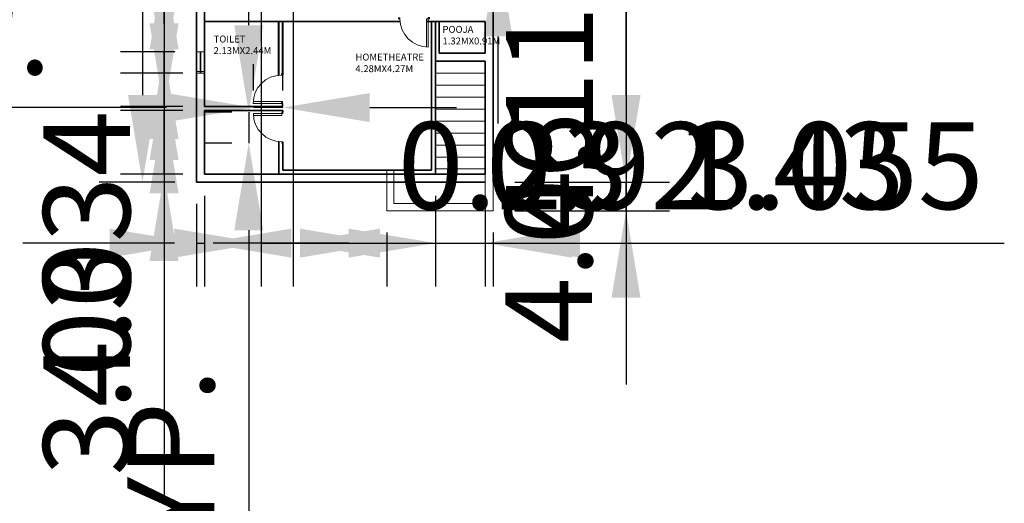
# Model space of a CAD drawing. Units: metres. Extents: x 1246 to 2549, y 2050 to 4184.
# Tile 3 of 6: x 1268 to 1297, y 2074 to 2088. Entities that reach past the tile are written whole.
import ezdxf

# ---------------------------------------------------------------- set-up
doc = ezdxf.new("R2010")
doc.units = ezdxf.units.M
for name, color, linetype, lineweight in [('A-ANNO-DIMS', 2, 'Continuous', 18), ('A-AREA-IDEN', 7, 'Continuous', 18), ('A-DOOR', 3, 'Continuous', 18), ('A-FLOR-STRS', 7, 'Continuous', 18), ('A-GLAZ', 4, 'Continuous', 18), ('A-WALL', 7, 'Continuous', 35)]:
    doc.layers.add(name, color=color, linetype=linetype, lineweight=lineweight)
doc.styles.get("Standard").update_dxf_attribs({"font": 'arial.ttf'})
doc.dimstyles.new('ISO-25', dxfattribs={"dimtxt": 2.5, "dimasz": 2.5, "dimexe": 1.25, "dimexo": 0.625, "dimtad": 1, "dimtxsty": 'Standard', "dimcen": 2.5, "dimadec": 0, "dimazin": 0, "dimtfac": 1, "dimtmove": 0, "dimatfit": 3, "dimfxl": 1, "dimarcsym": 0})

# ---------------------------------------------------------------- blocks, each defined once
blk = doc.blocks.new('*D2')
at = {"layer": 'A-ANNO-DIMS', "color": 0, "lineweight": -2, "transparency": 16777216}
for p, q in [((1272.709, 2100.209), (1270.53, 2100.209)), ((1271.78, 2097.709), (1271.78, 2086.022)), ((1272.709, 2083.522), (1270.53, 2083.522))]:
    blk.add_line(p, q, dxfattribs=at)
at = {"layer": 'A-ANNO-DIMS', "color": 0, "transparency": 16777216}
for points in [[(1271.364, 2097.709), (1272.197, 2097.709), (1271.78, 2100.209)], [(1271.364, 2086.022), (1272.197, 2086.022), (1271.78, 2083.522)]]:
    blk.add_solid(points, dxfattribs=at)
at = {"layer": 'Defpoints', "color": 0, "transparency": 16777216}
for p in [(1273.334, 2100.209), (1271.78, 2083.522), (1273.334, 2083.522)]:
    blk.add_point(p, dxfattribs=at)
at = {"layer": 'A-ANNO-DIMS', "color": 0, "transparency": 16777216, "insert": (1264.522, 2091.865), "char_height": 2.5, "attachment_point": 5, "rotation": 90}
blk.add_mtext('{\\H0.4x;\\P\\H0.5x;\\P\\P\\P\\P\\P\\P\\P 16,69}', dxfattribs=at)
blk = doc.blocks.new('DOOR-SWING-813')
for p, q in [((0.033, 0.039), (0.033, 0.09)), ((0.033, 0.09), (0.844, 0.09))]:
    blk.add_line(p, q)
for points in [[(0.033, 0.852), (0.033, 0.891), (0.002, 0.891), (0.002, 0.852)], [(0.033, 0.039), (0.033, 0), (0, 0), (0, 0.039)]]:
    blk.add_lwpolyline(points, close=True)
blk.add_lwpolyline([(0.846, 0.039), (0.033, 0.039), (0.033, 0.09)])
blk.add_arc((0.033, 0.039), 0.813, 0, 90)
blk = doc.blocks.new('*D7')
at = {"layer": 'A-ANNO-DIMS', "color": 0, "lineweight": -2, "transparency": 16777216}
for p, q in [((1274.837, 2088.031), (1274.837, 2090.531)), ((1274.346, 2085.531), (1273.587, 2085.531)), ((1274.837, 2085.531), (1274.837, 2084.639)), ((1274.346, 2084.639), (1273.587, 2084.639)), ((1274.837, 2082.139), (1274.837, 2049.849))]:
    blk.add_line(p, q, dxfattribs=at)
at = {"layer": 'A-ANNO-DIMS', "color": 0, "transparency": 16777216}
for points in [[(1274.421, 2088.031), (1275.254, 2088.031), (1274.837, 2085.531)], [(1274.421, 2082.139), (1275.254, 2082.139), (1274.837, 2084.639)]]:
    blk.add_solid(points, dxfattribs=at)
at = {"layer": 'Defpoints', "color": 0, "transparency": 16777216}
for p in [(1274.971, 2085.531), (1274.837, 2084.639), (1274.971, 2084.639)]:
    blk.add_point(p, dxfattribs=at)
at = {"layer": 'A-ANNO-DIMS', "color": 0, "transparency": 16777216, "insert": (1272.918, 2064.744), "char_height": 2.5, "attachment_point": 5, "rotation": 90}
blk.add_mtext('DOOR-813 1 TYP.', dxfattribs=at)
blk = doc.blocks.new('*D8')
at = {"layer": 'A-ANNO-DIMS', "color": 0, "lineweight": -2, "transparency": 16777216}
for p, q in [((1274.971, 2086.156), (1274.971, 2086.914)), ((1275.817, 2086.156), (1275.817, 2086.914)), ((1272.471, 2085.664), (1258.73, 2085.664)), ((1275.817, 2085.664), (1274.971, 2085.664)), ((1278.317, 2085.664), (1280.817, 2085.664))]:
    blk.add_line(p, q, dxfattribs=at)
at = {"layer": 'A-ANNO-DIMS', "color": 0, "transparency": 16777216}
for points in [[(1272.471, 2086.081), (1272.471, 2085.248), (1274.971, 2085.664)], [(1278.317, 2086.081), (1278.317, 2085.248), (1275.817, 2085.664)]]:
    blk.add_solid(points, dxfattribs=at)
at = {"layer": 'Defpoints', "color": 0, "transparency": 16777216}
for p in [(1274.971, 2085.664), (1274.971, 2085.531), (1275.817, 2085.531)]:
    blk.add_point(p, dxfattribs=at)
at = {"layer": 'A-ANNO-DIMS', "color": 0, "transparency": 16777216, "insert": (1264.35, 2087.545), "char_height": 2.5, "attachment_point": 5}
blk.add_mtext('1 TYP.', dxfattribs=at)
blk = doc.blocks.new('*D9')
at = {"layer": 'A-ANNO-DIMS', "color": 0, "lineweight": -2, "transparency": 16777216}
for p, q in [((1282.004, 2093.624), (1282.004, 2122.452)), ((1282.004, 2090.21), (1282.004, 2091.124)), ((1282.492, 2091.124), (1283.254, 2091.124)), ((1282.492, 2090.21), (1283.254, 2090.21)), ((1282.004, 2087.71), (1282.004, 2085.21))]:
    blk.add_line(p, q, dxfattribs=at)
at = {"layer": 'A-ANNO-DIMS', "color": 0, "transparency": 16777216}
for points in [[(1281.587, 2093.624), (1282.42, 2093.624), (1282.004, 2091.124)], [(1281.587, 2087.71), (1282.42, 2087.71), (1282.004, 2090.21)]]:
    blk.add_solid(points, dxfattribs=at)
at = {"layer": 'Defpoints', "color": 0, "transparency": 16777216}
for p in [(1281.867, 2091.124), (1282.004, 2091.124), (1281.867, 2090.21)]:
    blk.add_point(p, dxfattribs=at)
at = {"layer": 'A-ANNO-DIMS', "color": 0, "transparency": 16777216, "insert": (1280.102, 2109.288), "char_height": 2.5, "attachment_point": 5, "rotation": 90}
blk.add_mtext('WIN-914 1 TYP.', dxfattribs=at)
blk = doc.blocks.new('*D13')
at = {"layer": 'A-ANNO-DIMS', "color": 0, "lineweight": -2, "transparency": 16777216}
for p, q in [((1278.812, 2082.074), (1278.812, 2080.517)), ((1281.867, 2082.074), (1281.867, 2080.517)), ((1276.312, 2081.767), (1273.812, 2081.767)), ((1278.812, 2081.767), (1281.867, 2081.767)), ((1284.367, 2081.767), (1296.57, 2081.767))]:
    blk.add_line(p, q, dxfattribs=at)
at = {"layer": 'A-ANNO-DIMS', "color": 0, "transparency": 16777216}
for points in [[(1276.312, 2082.183), (1276.312, 2081.35), (1278.812, 2081.767)], [(1284.367, 2082.183), (1284.367, 2081.35), (1281.867, 2081.767)]]:
    blk.add_solid(points, dxfattribs=at)
at = {"layer": 'Defpoints', "color": 0, "transparency": 16777216}
for p in [(1278.812, 2082.699), (1281.867, 2082.699), (1281.867, 2081.767)]:
    blk.add_point(p, dxfattribs=at)
at = {"layer": 'A-ANNO-DIMS', "color": 0, "transparency": 16777216, "insert": (1291.719, 2083.669), "char_height": 2.5, "attachment_point": 5}
blk.add_mtext('3.055', dxfattribs=at)
blk = doc.blocks.new('*D14')
at = {"layer": 'A-ANNO-DIMS', "color": 0, "lineweight": -2, "transparency": 16777216}
for p, q in [((1285.689, 2086.022), (1285.689, 2096.24)), ((1282.492, 2083.522), (1286.939, 2083.522)), ((1285.689, 2082.699), (1285.689, 2083.522)), ((1282.492, 2082.699), (1286.939, 2082.699)), ((1285.689, 2080.199), (1285.689, 2077.699))]:
    blk.add_line(p, q, dxfattribs=at)
at = {"layer": 'A-ANNO-DIMS', "color": 0, "transparency": 16777216}
for points in [[(1285.272, 2086.022), (1286.106, 2086.022), (1285.689, 2083.522)], [(1285.272, 2080.199), (1286.106, 2080.199), (1285.689, 2082.699)]]:
    blk.add_solid(points, dxfattribs=at)
at = {"layer": 'Defpoints', "color": 0, "transparency": 16777216}
for p in [(1281.867, 2083.522), (1285.689, 2083.522), (1281.867, 2082.699)]:
    blk.add_point(p, dxfattribs=at)
at = {"layer": 'A-ANNO-DIMS', "color": 0, "transparency": 16777216, "insert": (1283.788, 2092.381), "char_height": 2.5, "attachment_point": 5, "rotation": 90}
blk.add_mtext('0.82', dxfattribs=at)
blk = doc.blocks.new('*D15')
at = {"layer": 'A-ANNO-DIMS', "color": 0, "lineweight": -2, "transparency": 16777216}
for p, q in [((1272.401, 2088.082), (1272.401, 2098.09)), ((1272.939, 2085.582), (1271.151, 2085.582)), ((1272.401, 2083.752), (1272.401, 2085.582)), ((1272.939, 2083.752), (1271.151, 2083.752)), ((1272.401, 2081.252), (1272.401, 2078.752))]:
    blk.add_line(p, q, dxfattribs=at)
at = {"layer": 'A-ANNO-DIMS', "color": 0, "transparency": 16777216}
for points in [[(1271.985, 2088.082), (1272.818, 2088.082), (1272.401, 2085.582)], [(1271.985, 2081.252), (1272.818, 2081.252), (1272.401, 2083.752)]]:
    blk.add_solid(points, dxfattribs=at)
at = {"layer": 'Defpoints', "color": 0, "transparency": 16777216}
for p in [(1272.401, 2085.582), (1273.564, 2085.582), (1273.564, 2083.752)]:
    blk.add_point(p, dxfattribs=at)
at = {"layer": 'A-ANNO-DIMS', "color": 0, "transparency": 16777216, "insert": (1270.499, 2094.336), "char_height": 2.5, "attachment_point": 5, "rotation": 90}
blk.add_mtext('1.83', dxfattribs=at)
blk = doc.blocks.new('*D16')
at = {"layer": 'A-ANNO-DIMS', "color": 0, "lineweight": -2, "transparency": 16777216}
for p, q in [((1280.211, 2083.127), (1280.211, 2080.517)), ((1281.637, 2083.127), (1281.637, 2080.517)), ((1277.711, 2081.767), (1275.211, 2081.767)), ((1280.211, 2081.767), (1281.637, 2081.767)), ((1284.137, 2081.767), (1294.145, 2081.767))]:
    blk.add_line(p, q, dxfattribs=at)
at = {"layer": 'A-ANNO-DIMS', "color": 0, "transparency": 16777216}
for points in [[(1277.711, 2082.183), (1277.711, 2081.35), (1280.211, 2081.767)], [(1284.137, 2082.183), (1284.137, 2081.35), (1281.637, 2081.767)]]:
    blk.add_solid(points, dxfattribs=at)
at = {"layer": 'Defpoints', "color": 0, "transparency": 16777216}
for p in [(1280.211, 2083.752), (1281.637, 2083.752), (1281.637, 2081.767)]:
    blk.add_point(p, dxfattribs=at)
at = {"layer": 'A-ANNO-DIMS', "color": 0, "transparency": 16777216, "insert": (1290.391, 2083.669), "char_height": 2.5, "attachment_point": 5}
blk.add_mtext('1.43', dxfattribs=at)
blk = doc.blocks.new('*D17')
at = {"layer": 'A-ANNO-DIMS', "color": 0, "lineweight": -2, "transparency": 16777216}
for p, q in [((1275.198, 2099.354), (1275.198, 2080.517)), ((1276.114, 2099.356), (1276.114, 2080.517)), ((1272.698, 2081.767), (1270.198, 2081.767)), ((1275.198, 2081.767), (1276.114, 2081.767)), ((1278.614, 2081.767), (1288.832, 2081.767))]:
    blk.add_line(p, q, dxfattribs=at)
at = {"layer": 'A-ANNO-DIMS', "color": 0, "transparency": 16777216}
for points in [[(1272.698, 2082.183), (1272.698, 2081.35), (1275.198, 2081.767)], [(1278.614, 2082.183), (1278.614, 2081.35), (1276.114, 2081.767)]]:
    blk.add_solid(points, dxfattribs=at)
at = {"layer": 'Defpoints', "color": 0, "transparency": 16777216}
for p in [(1275.198, 2099.979), (1276.114, 2099.981), (1276.114, 2081.767)]:
    blk.add_point(p, dxfattribs=at)
at = {"layer": 'A-ANNO-DIMS', "color": 0, "transparency": 16777216, "insert": (1284.973, 2083.668), "char_height": 2.5, "attachment_point": 5}
blk.add_mtext('0.92', dxfattribs=at)
blk = doc.blocks.new('*D19')
at = {"layer": 'A-ANNO-DIMS', "color": 0, "lineweight": -2, "transparency": 16777216}
for p, q in [((1285.689, 2102.709), (1285.689, 2105.209)), ((1282.492, 2100.209), (1286.939, 2100.209)), ((1285.689, 2100.209), (1285.689, 2096.096)), ((1282.492, 2096.096), (1286.939, 2096.096)), ((1285.689, 2093.596), (1285.689, 2081.335))]:
    blk.add_line(p, q, dxfattribs=at)
at = {"layer": 'A-ANNO-DIMS', "color": 0, "transparency": 16777216}
for points in [[(1285.272, 2102.709), (1286.106, 2102.709), (1285.689, 2100.209)], [(1285.272, 2093.596), (1286.106, 2093.596), (1285.689, 2096.096)]]:
    blk.add_solid(points, dxfattribs=at)
at = {"layer": 'Defpoints', "color": 0, "transparency": 16777216}
for p in [(1281.867, 2100.209), (1281.867, 2096.096), (1285.689, 2096.096)]:
    blk.add_point(p, dxfattribs=at)
at = {"layer": 'A-ANNO-DIMS', "color": 0, "transparency": 16777216, "insert": (1283.809, 2086.216), "char_height": 2.5, "attachment_point": 5, "rotation": 90}
blk.add_mtext('4.112', dxfattribs=at)
blk = doc.blocks.new('*D20')
at = {"layer": 'A-ANNO-DIMS', "color": 0, "lineweight": -2, "transparency": 16777216}
for p, q in [((1285.689, 2097.682), (1285.689, 2100.182)), ((1282.492, 2095.182), (1286.939, 2095.182)), ((1285.689, 2095.182), (1285.689, 2091.124)), ((1282.492, 2091.124), (1286.939, 2091.124)), ((1285.689, 2088.624), (1285.689, 2078.281))]:
    blk.add_line(p, q, dxfattribs=at)
at = {"layer": 'A-ANNO-DIMS', "color": 0, "transparency": 16777216}
for points in [[(1285.272, 2097.682), (1286.106, 2097.682), (1285.689, 2095.182)], [(1285.272, 2088.624), (1286.106, 2088.624), (1285.689, 2091.124)]]:
    blk.add_solid(points, dxfattribs=at)
at = {"layer": 'Defpoints', "color": 0, "transparency": 16777216}
for p in [(1281.867, 2095.182), (1281.867, 2091.124), (1285.689, 2091.124)]:
    blk.add_point(p, dxfattribs=at)
at = {"layer": 'A-ANNO-DIMS', "color": 0, "transparency": 16777216, "insert": (1283.788, 2082.203), "char_height": 2.5, "attachment_point": 5, "rotation": 90}
blk.add_mtext('4.06', dxfattribs=at)
blk = doc.blocks.new('*D21')
at = {"layer": 'A-ANNO-DIMS', "color": 0, "lineweight": -2, "transparency": 16777216}
for p, q in [((1272.401, 2097.74), (1272.401, 2100.24)), ((1272.709, 2095.24), (1271.151, 2095.24)), ((1272.401, 2095.24), (1272.401, 2091.205)), ((1272.711, 2091.205), (1271.151, 2091.205)), ((1272.401, 2088.705), (1272.401, 2076.429))]:
    blk.add_line(p, q, dxfattribs=at)
at = {"layer": 'A-ANNO-DIMS', "color": 0, "transparency": 16777216}
for points in [[(1271.985, 2097.74), (1272.818, 2097.74), (1272.401, 2095.24)], [(1271.985, 2088.705), (1272.818, 2088.705), (1272.401, 2091.205)]]:
    blk.add_solid(points, dxfattribs=at)
at = {"layer": 'Defpoints', "color": 0, "transparency": 16777216}
for p in [(1273.334, 2095.24), (1272.401, 2091.205), (1273.336, 2091.205)]:
    blk.add_point(p, dxfattribs=at)
at = {"layer": 'A-ANNO-DIMS', "color": 0, "transparency": 16777216, "insert": (1270.499, 2081.317), "char_height": 2.5, "attachment_point": 5, "rotation": 90}
blk.add_mtext('4.034', dxfattribs=at)
blk = doc.blocks.new('*D22')
at = {"layer": 'A-ANNO-DIMS', "color": 0, "lineweight": -2, "transparency": 16777216}
for p, q in [((1272.401, 2092.791), (1272.401, 2095.291)), ((1272.711, 2090.291), (1271.151, 2090.291)), ((1272.401, 2090.291), (1272.401, 2087.264)), ((1272.708, 2087.264), (1271.151, 2087.264)), ((1272.401, 2084.764), (1272.401, 2074.522))]:
    blk.add_line(p, q, dxfattribs=at)
at = {"layer": 'A-ANNO-DIMS', "color": 0, "transparency": 16777216}
for points in [[(1271.985, 2092.791), (1272.818, 2092.791), (1272.401, 2090.291)], [(1271.985, 2084.764), (1272.818, 2084.764), (1272.401, 2087.264)]]:
    blk.add_solid(points, dxfattribs=at)
at = {"layer": 'Defpoints', "color": 0, "transparency": 16777216}
for p in [(1273.336, 2090.291), (1272.401, 2087.264), (1273.333, 2087.264)]:
    blk.add_point(p, dxfattribs=at)
at = {"layer": 'A-ANNO-DIMS', "color": 0, "transparency": 16777216, "insert": (1270.499, 2078.393), "char_height": 2.5, "attachment_point": 5, "rotation": 90}
blk.add_mtext('3.03', dxfattribs=at)
blk = doc.blocks.new('*D25')
at = {"layer": 'A-ANNO-DIMS', "color": 0, "lineweight": -2, "transparency": 16777216}
for p, q in [((1272.401, 2094.497), (1272.401, 2104.781)), ((1275.811, 2091.997), (1271.151, 2091.997)), ((1272.401, 2089.84), (1272.401, 2091.997)), ((1275.811, 2089.84), (1271.151, 2089.84)), ((1272.401, 2087.34), (1272.401, 2084.84))]:
    blk.add_line(p, q, dxfattribs=at)
at = {"layer": 'A-ANNO-DIMS', "color": 0, "transparency": 16777216}
for points in [[(1271.985, 2094.497), (1272.818, 2094.497), (1272.401, 2091.997)], [(1271.985, 2087.34), (1272.818, 2087.34), (1272.401, 2089.84)]]:
    blk.add_solid(points, dxfattribs=at)
at = {"layer": 'Defpoints', "color": 0, "transparency": 16777216}
for p in [(1272.401, 2091.997), (1276.436, 2091.997), (1276.436, 2089.84)]:
    blk.add_point(p, dxfattribs=at)
at = {"layer": 'A-ANNO-DIMS', "color": 0, "transparency": 16777216, "insert": (1270.5, 2100.889), "char_height": 2.5, "attachment_point": 5, "rotation": 90}
blk.add_mtext('2.16', dxfattribs=at)
blk = doc.blocks.new('*D26')
at = {"layer": 'A-ANNO-DIMS', "color": 0, "lineweight": -2, "transparency": 16777216}
for p, q in [((1273.564, 2083.127), (1273.564, 2080.517)), ((1273.334, 2082.897), (1273.334, 2080.517)), ((1270.834, 2081.767), (1268.334, 2081.767)), ((1273.334, 2081.767), (1273.564, 2081.767)), ((1276.064, 2081.767), (1286.308, 2081.767))]:
    blk.add_line(p, q, dxfattribs=at)
at = {"layer": 'A-ANNO-DIMS', "color": 0, "transparency": 16777216}
for points in [[(1270.834, 2082.183), (1270.834, 2081.35), (1273.334, 2081.767)], [(1276.064, 2082.183), (1276.064, 2081.35), (1273.564, 2081.767)]]:
    blk.add_solid(points, dxfattribs=at)
at = {"layer": 'Defpoints', "color": 0, "transparency": 16777216}
for p in [(1273.564, 2083.752), (1273.334, 2083.522), (1273.564, 2081.767)]:
    blk.add_point(p, dxfattribs=at)
at = {"layer": 'A-ANNO-DIMS', "color": 0, "transparency": 16777216, "insert": (1282.436, 2083.669), "char_height": 2.5, "attachment_point": 5}
blk.add_mtext('0.23', dxfattribs=at)
blk = doc.blocks.new('*D28')
at = {"layer": 'A-ANNO-DIMS', "color": 0, "lineweight": -2, "transparency": 16777216}
for p, q in [((1272.401, 2089.155), (1272.401, 2099.397)), ((1272.938, 2086.655), (1271.151, 2086.655)), ((1272.401, 2085.696), (1272.401, 2086.655)), ((1272.939, 2085.696), (1271.151, 2085.696)), ((1272.401, 2083.196), (1272.401, 2080.696))]:
    blk.add_line(p, q, dxfattribs=at)
at = {"layer": 'A-ANNO-DIMS', "color": 0, "transparency": 16777216}
for points in [[(1271.985, 2089.155), (1272.818, 2089.155), (1272.401, 2086.655)], [(1271.985, 2083.196), (1272.818, 2083.196), (1272.401, 2085.696)]]:
    blk.add_solid(points, dxfattribs=at)
at = {"layer": 'Defpoints', "color": 0, "transparency": 16777216}
for p in [(1272.401, 2086.655), (1273.563, 2086.655), (1273.564, 2085.696)]:
    blk.add_point(p, dxfattribs=at)
at = {"layer": 'A-ANNO-DIMS', "color": 0, "transparency": 16777216, "insert": (1270.5, 2095.526), "char_height": 2.5, "attachment_point": 5, "rotation": 90}
blk.add_mtext('0.96', dxfattribs=at)
blk = doc.blocks.new('*D29')
at = {"layer": 'A-ANNO-DIMS', "color": 0, "lineweight": -2, "transparency": 16777216}
for p, q in [((1272.401, 2089.764), (1272.401, 2099.525)), ((1272.708, 2087.264), (1271.151, 2087.264)), ((1272.401, 2086.655), (1272.401, 2087.264)), ((1272.708, 2086.655), (1271.151, 2086.655)), ((1272.401, 2084.155), (1272.401, 2081.655))]:
    blk.add_line(p, q, dxfattribs=at)
at = {"layer": 'A-ANNO-DIMS', "color": 0, "transparency": 16777216}
for points in [[(1271.985, 2089.764), (1272.818, 2089.764), (1272.401, 2087.264)], [(1271.985, 2084.155), (1272.818, 2084.155), (1272.401, 2086.655)]]:
    blk.add_solid(points, dxfattribs=at)
at = {"layer": 'Defpoints', "color": 0, "transparency": 16777216}
for p in [(1272.401, 2087.264), (1273.333, 2087.264), (1273.333, 2086.655)]:
    blk.add_point(p, dxfattribs=at)
at = {"layer": 'A-ANNO-DIMS', "color": 0, "transparency": 16777216, "insert": (1270.5, 2095.894), "char_height": 2.5, "attachment_point": 5, "rotation": 90}
blk.add_mtext('0.61', dxfattribs=at)

msp = doc.modelspace()

# ---------------------------------------------------------------- linework, layer by layer
at = {"layer": 'A-DOOR'}
for p, q in [((1275.7752, 2085.836), (1274.964, 2085.836)), ((1275.7752, 2085.7852), (1275.7752, 2085.836)), ((1275.7752, 2085.836), (1275.8083, 2085.836)), ((1275.7752, 2085.7852), (1275.8083, 2085.7852)), ((1275.8083, 2085.836), (1275.8083, 2085.7852))]:
    msp.add_line(p, q, dxfattribs=at)
msp.add_lwpolyline([(1275.7752, 2086.598), (1275.7752, 2086.6379), (1275.8066, 2086.6379), (1275.8066, 2086.598)], close=True, dxfattribs=at)
msp.add_lwpolyline([(1274.9624, 2085.7852), (1275.7752, 2085.7852), (1275.7752, 2085.836)], dxfattribs=at)
msp.add_arc((1275.7752, 2085.7852), 0.8128, 90, 180, dxfattribs=at)
at = {"layer": 'A-FLOR-STRS'}
for p, q in [((1281.6369, 2086.9959), (1280.2112, 2086.9959)), ((1281.6369, 2086.6518), (1280.2112, 2086.6518)), ((1281.6369, 2086.3077), (1280.2112, 2086.3077)), ((1281.6369, 2085.9636), (1280.2112, 2085.9636)), ((1281.6369, 2085.6195), (1280.2112, 2085.6195)), ((1281.6369, 2085.2755), (1280.2112, 2085.2755)), ((1281.6369, 2084.9314), (1280.2112, 2084.9314)), ((1281.6369, 2084.5873), (1280.2112, 2084.5873)), ((1281.6369, 2084.2432), (1280.2112, 2084.2432)), ((1278.8119, 2083.5216), (1278.8119, 2083.8659)), ((1279.0119, 2083.5216), (1279.0119, 2083.8659)), ((1281.6369, 2083.8991), (1280.2112, 2083.8991)), ((1281.6369, 2083.7516), (1281.6369, 2082.9092)), ((1278.8119, 2082.6987), (1278.8119, 2083.5216)), ((1279.0119, 2082.9092), (1279.0119, 2083.5216)), ((1281.8669, 2083.5216), (1281.8669, 2082.6987)), ((1281.6369, 2082.9092), (1279.0119, 2082.9092)), ((1281.8669, 2082.6987), (1278.8119, 2082.6987))]:
    msp.add_line(p, q, dxfattribs=at)
at = {"layer": 'A-GLAZ'}
for p, q in [((1273.3333, 2086.6546), (1273.3333, 2087.2638)), ((1273.3333, 2087.2638), (1273.5633, 2087.2638)), ((1273.4356, 2086.6546), (1273.4356, 2087.2638)), ((1273.4483, 2086.6546), (1273.4483, 2087.2638)), ((1273.461, 2086.6546), (1273.461, 2087.2638)), ((1273.5633, 2087.2638), (1273.5633, 2086.6546)), ((1273.5633, 2087.2638), (1273.5633, 2087.213)), ((1273.5633, 2086.7054), (1273.3333, 2086.7054)), ((1273.5633, 2086.6546), (1273.3333, 2086.6546)), ((1273.5633, 2086.6546), (1273.5633, 2086.7054))]:
    msp.add_line(p, q, dxfattribs=at)
at = {"layer": 'A-WALL'}
for p, q in [((1273.334, 2093.2445), (1273.334, 2088.1359)), ((1273.564, 2093.1302), (1273.564, 2088.1359)), ((1281.8669, 2087.9121), (1281.8669, 2088.4556)), ((1273.334, 2088.1359), (1273.334, 2085.6959)), ((1273.564, 2088.1359), (1275.8169, 2088.1359)), ((1273.564, 2088.1359), (1273.564, 2085.6959)), ((1275.694, 2086.5939), (1275.694, 2088.1359)), ((1275.7026, 2086.5947), (1275.7026, 2088.1359)), ((1275.8083, 2086.5973), (1275.8083, 2088.1359)), ((1275.8169, 2088.1359), (1279.1917, 2088.1359)), ((1279.1917, 2088.1359), (1275.8169, 2088.1359)), ((1275.8169, 2086.5969), (1275.8169, 2088.1359)), ((1281.6369, 2088.1359), (1279.9496, 2088.1359)), ((1279.9496, 2088.1359), (1280.0969, 2088.1359)), ((1280.0969, 2088.1359), (1280.0969, 2083.8659)), ((1280.2112, 2088.1359), (1280.2112, 2083.7516)), ((1280.2112, 2088.1359), (1281.5312, 2088.1359)), ((1281.6369, 2088.1359), (1280.3169, 2088.1359)), ((1280.3169, 2088.1359), (1280.3169, 2087.2259)), ((1281.6369, 2087.2259), (1281.6369, 2088.1359)), ((1281.8669, 2087.2259), (1281.8669, 2087.9121)), ((1280.3169, 2087.2259), (1281.6369, 2087.2259)), ((1281.8669, 2087.2259), (1281.8669, 2083.5216)), ((1280.2112, 2086.9959), (1281.6369, 2086.9959)), ((1281.6369, 2086.9959), (1281.6369, 2083.7516)), ((1273.334, 2085.6959), (1273.334, 2083.5216)), ((1273.564, 2085.6959), (1275.694, 2085.6959)), ((1275.694, 2085.6959), (1275.8083, 2085.6959)), ((1275.8083, 2085.6959), (1275.8083, 2085.7852)), ((1275.8083, 2085.6959), (1275.8083, 2085.7467)), ((1273.564, 2085.5816), (1275.694, 2085.5816)), ((1273.564, 2085.5816), (1273.564, 2083.7516)), ((1275.694, 2085.5816), (1275.8169, 2085.5816)), ((1275.8169, 2085.5816), (1275.8169, 2085.5308)), ((1275.7026, 2083.8659), (1275.7026, 2084.6835)), ((1275.8169, 2083.8659), (1275.8169, 2084.6801)), ((1273.564, 2083.7516), (1275.8083, 2083.7516)), ((1275.7026, 2083.7516), (1275.7026, 2083.8659)), ((1280.0969, 2083.8659), (1275.8169, 2083.8659)), ((1280.0969, 2083.7516), (1275.8169, 2083.7516)), ((1281.6369, 2083.7516), (1280.0969, 2083.7516)), ((1273.334, 2083.5216), (1275.8083, 2083.5216)), ((1280.0969, 2083.5216), (1275.8169, 2083.5216)), ((1281.6369, 2083.5216), (1280.0969, 2083.5216))]:
    msp.add_line(p, q, dxfattribs=at)

# ---------------------------------------------------------------- block references
at = {"layer": 'A-DOOR', "extrusion": (0, 0, -1), "zscale": -1, "rotation": 270.0000000000915}
msp.add_blockref('DOOR-SWING-813', (-1280.0392, 2088.2502), dxfattribs=at)
at = {"layer": 'A-DOOR', "rotation": 180}
msp.add_blockref('DOOR-SWING-813', (1275.817, 2085.531), dxfattribs=at)

# ---------------------------------------------------------------- texts
at = {"layer": 'A-AREA-IDEN', "char_height": 0.5, "attachment_point": 1}
for s, heights, insert in [('{\\H0.4x;POOJA\\P1.32MX0.91M}', [0], (1280.41, 2088.0123)), ('{\\H0.4x;TOILET\\P2.13MX2.44M}', [0], (1273.826, 2087.7354)), ('{\\H0.4x;HOMETHEATRE\\P4.28MX4.27M}', [1.0744], (1277.9058, 2087.2165))]:
    msp.add_mtext_dynamic_manual_height_columns(s, width=2.167266, gutter_width=12.5, heights=heights, dxfattribs=dict(at, insert=insert))

# ---------------------------------------------------------------- dimensions: what is measured, and where the dimension line sits
at = {"layer": 'A-ANNO-DIMS'}
for base, p1, p2, angle, text, override, picture, middle in [((1282.0037, 2091.1239), (1281.8666, 2090.2099), (1281.8666, 2091.1239), 90, 'WIN-914 <> TYP.', {"dimdec": 0, "dimlfac": 1, "dimrnd": 0, "dimzin": 0, "dimdsep": 46, "dimlunit": 2}, '*D9', (1280.1022, 2109.2881)), ((1271.7804, 2083.5216), (1273.334, 2100.2088), (1273.334, 2083.5216), 90, '{\\H0.4x;\\P\\H0.5x;\\P\\P\\P\\P\\P\\P\\P <>}', {"dimclrd": 0, "dimclre": 0, "dimclrt": 0}, '*D2', (1264.5216, 2091.8652)), ((1274.971, 2085.6644), (1275.8169, 2085.5308), (1274.971, 2085.5308), 180, '<> TYP.', {"dimdec": 0, "dimlfac": 1, "dimrnd": 0, "dimzin": 0, "dimdsep": 46, "dimlunit": 2}, '*D8', (1264.3503, 2087.5454)), ((1274.8373, 2084.6395), (1274.971, 2085.5308), (1274.971, 2084.6395), 270, 'DOOR-813 <> TYP.', {"dimdec": 0, "dimlfac": 1, "dimrnd": 0, "dimzin": 0, "dimdsep": 46, "dimlunit": 2}, '*D7', (1272.918, 2064.7444))]:
    dim = msp.add_linear_dim(base=base, p1=p1, p2=p2, angle=angle, text=text, dimstyle='ISO-25', override=override, dxfattribs=at)
    dim.commit()
    dim.dimension.update_dxf_attribs({"geometry": picture, "text_midpoint": middle})
for base, p1, p2, override, picture, middle in [((1285.689, 2096.0964), (1281.8669, 2100.2088), (1281.8668, 2096.0964), {"dimdec": 3, "dimlfac": 1, "dimrnd": 0, "dimzin": 0, "dimdsep": 46, "dimlunit": 2}, '*D19', (1283.8089, 2086.2158)), ((1272.4013, 2091.9965), (1276.4362, 2089.8402), (1276.4362, 2091.9965), {"dimdec": 2, "dimlfac": 1, "dimrnd": 0, "dimzin": 0, "dimdsep": 46, "dimlunit": 2}, '*D25', (1270.4999, 2100.8889)), ((1272.4013, 2091.2053), (1273.3339, 2095.2396), (1273.3356, 2091.2053), {"dimdec": 3, "dimlfac": 1, "dimrnd": 0, "dimzin": 0, "dimdsep": 46, "dimlunit": 2}, '*D21', (1270.499, 2081.317)), ((1285.689, 2091.1239), (1281.8668, 2095.1824), (1281.8666, 2091.1239), {"dimdec": 2, "dimlfac": 1, "dimrnd": 0, "dimzin": 0, "dimdsep": 46, "dimlunit": 2}, '*D20', (1283.7876, 2082.2025)), ((1272.4013, 2087.2638), (1273.3333, 2086.6546), (1273.3333, 2087.2638), {"dimdec": 2, "dimlfac": 1, "dimrnd": 0, "dimzin": 0, "dimdsep": 46, "dimlunit": 2}, '*D29', (1270.4999, 2095.8944)), ((1272.4013, 2086.6546), (1273.564, 2085.6959), (1273.5633, 2086.6546), {"dimdec": 2, "dimlfac": 1, "dimrnd": 0, "dimzin": 0, "dimdsep": 46, "dimlunit": 2}, '*D28', (1270.4999, 2095.5257)), ((1272.4013, 2085.5816), (1273.564, 2083.7516), (1273.564, 2085.5816), {"dimdec": 2, "dimlfac": 1, "dimrnd": 0, "dimzin": 0, "dimdsep": 46, "dimlunit": 2}, '*D15', (1270.499, 2094.3358)), ((1285.689, 2083.5216), (1281.8669, 2082.6987), (1281.8669, 2083.5216), {"dimdec": 2, "dimlfac": 1, "dimrnd": 0, "dimzin": 0, "dimdsep": 46, "dimlunit": 2}, '*D14', (1283.7876, 2092.3807)), ((1272.4013, 2087.2638), (1273.3356, 2090.2913), (1273.3333, 2087.2638), {"dimdec": 2, "dimlfac": 1, "dimrnd": 0, "dimzin": 0, "dimdsep": 46, "dimlunit": 2}, '*D22', (1270.499, 2078.3927))]:
    dim = msp.add_linear_dim(base=base, p1=p1, p2=p2, angle=90, dimstyle='ISO-25', override=override, dxfattribs=at)
    dim.commit()
    dim.dimension.update_dxf_attribs({"geometry": picture, "text_midpoint": middle})
for base, p1, p2, override, picture, middle in [((1276.1137, 2081.7667), (1275.1983, 2099.9788), (1276.1137, 2099.9811), {"dimdec": 2, "dimlfac": 1, "dimrnd": 0, "dimzin": 0, "dimdsep": 46, "dimlunit": 2}, '*D17', (1284.9729, 2083.6681)), ((1273.564, 2081.7667), (1273.334, 2083.5216), (1273.564, 2083.7516), {"dimdec": 2, "dimlfac": 1, "dimrnd": 0, "dimzin": 0, "dimdsep": 46, "dimlunit": 2}, '*D26', (1282.436, 2083.669)), ((1281.8669, 2081.7667), (1278.8119, 2082.6987), (1281.8669, 2082.6987), {"dimdec": 3, "dimlfac": 1, "dimrnd": 0, "dimzin": 0, "dimdsep": 46, "dimlunit": 2}, '*D13', (1291.7186, 2083.669)), ((1281.6369, 2081.7667), (1280.2112, 2083.7516), (1281.6369, 2083.7516), {"dimdec": 2, "dimlfac": 1, "dimrnd": 0, "dimzin": 0, "dimdsep": 46, "dimlunit": 2}, '*D16', (1290.3912, 2083.669))]:
    dim = msp.add_linear_dim(base=base, p1=p1, p2=p2, dimstyle='ISO-25', override=override, dxfattribs=at)
    dim.commit()
    dim.dimension.update_dxf_attribs({"geometry": picture, "text_midpoint": middle})

doc.saveas('drawing.dxf')
